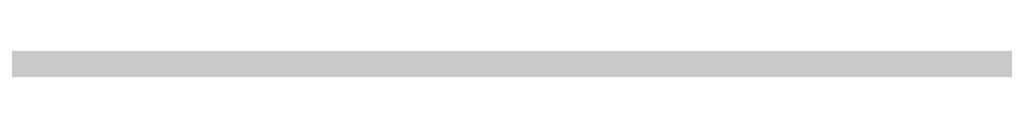
# Model space of a CAD drawing. Units: inches. Extents: x 2091 to 2899, y 967 to 2217.
# Tile 227 of 256: x 2203.4104 to 2203.7172, y 1152.2504 to 1152.2538. Entities that reach past the tile are written whole.
import ezdxf

# ---------------------------------------------------------------- set-up
doc = ezdxf.new("R2010")
doc.units = ezdxf.units.IN
doc.layers.add('A-WALL-PATT', color=141, linetype='Continuous', lineweight=13, true_color=0xadddf7)

msp = doc.modelspace()

# ---------------------------------------------------------------- hatches: boundary and pattern name
at = {"layer": 'A-WALL-PATT'}
h = msp.add_hatch(color=256, dxfattribs=at)
h.dxf.hatch_style = 1
h.paths.add_polyline_path([(2803.1436, 2050.91906), (2203.1436, 2050.91906), (2203.1436, 1090.91906), (2803.1436, 1090.91906)])
h.paths.add_polyline_path([(2635.79885, 1147.54046), (2674.52405, 1147.54046, 0.376086), (2678.52967, 1152.8802), (2678.52967, 1159.55647, 0.333335), (2674.52432, 1163.56185), (2674.52432, 1163.56185), (2674.52432, 1192.93439), (2635.80597, 1192.93439), (2597.08762, 1192.93439), (2597.08762, 1163.56185, 0.333335), (2593.08228, 1159.55647), (2593.08228, 1152.8802, 0.376086), (2597.08789, 1147.54046)], flags=0)
h.paths.add_polyline_path([(2436.01043, 1278.24078, 0.000483), (2435.95264, 1278.21503, -0.001328), (2435.93563, 1278.11169, -0.001711), (2436.11644, 1278.04076, 0.002185)], flags=0)
h.paths.add_polyline_path([(2794.1436, 1143.41906), (2794.1436, 1347.41906), (2543.37017, 1347.41906), (2543.37017, 1351.91906), (2794.1436, 1351.91906), (2794.1436, 1392.71355), (2793.9474, 1392.71355), (2793.9474, 1473.5369), (2794.1436, 1473.5369), (2794.1436, 1531.91906), (2650.1436, 1531.91906), (2650.1436, 1536.41906), (2794.1436, 1536.41906), (2794.1436, 1692.41906), (2609.37561, 1692.41906), (2609.37561, 1644.41906), (2604.87561, 1644.41906), (2604.87561, 1744.91906), (2609.37561, 1744.91906), (2609.37561, 1696.91906), (2794.1436, 1696.91906), (2794.1436, 1780.91906), (2609.6436, 1780.91906), (2493.87561, 1780.91906), (2493.87561, 1785.41906), (2609.6436, 1785.41906), (2794.1436, 1785.41906), (2794.1436, 1847.93882), (2793.95122, 1847.93882), (2793.95122, 1928.76217), (2794.1436, 1928.76217), (2794.1436, 1941.41906), (2614.1436, 1941.41906), (2614.1436, 1821.41906), (2609.6436, 1821.41906), (2609.6436, 1941.41906), (2392.1436, 1941.41906), (2392.1436, 1819.91906), (2387.6436, 1819.91906), (2387.6436, 1941.41906), (2212.1436, 1941.41906), (2212.1436, 1783.91906), (2392.1436, 1783.91906), (2392.1436, 1780.91906), (2212.1436, 1780.91906), (2212.1436, 1629.41906), (2387.6436, 1629.41906), (2387.6436, 1744.91906), (2392.1436, 1744.91906), (2392.1436, 1627.91906), (2317.1436, 1627.91906), (2317.1436, 1551.41906), (2317.1436, 1536.41906), (2459.38359, 1536.41906), (2459.38359, 1602.39648), (2463.88359, 1602.39648), (2463.88359, 1531.91906), (2456.6436, 1531.91906), (2456.6436, 1529.91906), (2452.1436, 1529.91906), (2452.1436, 1531.91906), (2312.6436, 1531.91906), (2312.6436, 1551.41906), (2306.1436, 1551.41906), (2306.1436, 1555.91906), (2308.1436, 1555.91906), (2308.1436, 1551.41906), (2312.6436, 1551.41906), (2312.6436, 1627.91906), (2212.1436, 1627.91906), (2212.1436, 1555.91906), (2270.1436, 1555.91906), (2270.1436, 1551.41906), (2212.1436, 1551.41906), (2212.1436, 1351.91906), (2272.1436, 1351.91906), (2272.1436, 1347.41906), (2212.1436, 1347.41906), (2212.1436, 1275.41906), (2308.1436, 1275.41906), (2308.1436, 1351.91906), (2452.1436, 1351.91906), (2452.1436, 1493.91906), (2456.6436, 1493.91906), (2456.6436, 1347.41906), (2312.6436, 1347.41906), (2312.6436, 1270.91906), (2212.1436, 1270.91906), (2212.1436, 1099.91906), (2281.23752, 1099.91906), (2282.87104, 1110.9138), (2282.00834, 1116.9966), (2278.55774, 1121.4204), (2268.20564, 1128.0562), (2272.08764, 1128.0562), (2273.81294, 1131.927), (2279.42034, 1134.6919), (2285.02784, 1135.2449), (2287.61584, 1137.4568), (2288.04714, 1138.0098), (2289.34114, 1140.7747), (2291.06654, 1139.6687), (2292.36054, 1135.2449), (2295.37984, 1136.9038), (2296.24254, 1135.7979), (2297.10524, 1133.033), (2300.12464, 1138.0098), (2303.14394, 1138.0098), (2304.43794, 1135.7979), (2303.14394, 1133.586), (2306.59464, 1134.6919), (2307.88874, 1133.033), (2310.90804, 1135.2449), (2313.92744, 1134.1389), (2315.62686, 1132.4271), (2308.32004, 1117.5496), (2290.20384, 1109.8079), (2288.90984, 1103.1721), (2289.27231, 1099.91906), (2434.91823, 1099.91906), (2431.59323, 1124.78806), (2429.93023, 1169.55306), (2430.92718, 1240.51969), (2435.65893, 1238.18613), (2437.13523, 1196.55406), (2438.79823, 1143.97306), (2442.67823, 1111.99806), (2446.55823, 1099.91906), (2794.1436, 1099.91906), (2794.1436, 1138.91906), (2548.03245, 1138.91906), (2548.03245, 1143.41906), (2548.03245, 1148.81906), (2546.66846, 1148.03156), (2528.68569, 1179.17862, 0.256256), (2512.03245, 1148.81906), (2512.03245, 1143.41906), (2512.03245, 1138.91906), (2507.53245, 1138.91906), (2507.53245, 1143.41906), (2507.53245, 1148.81906, 0.256256), (2490.8792, 1179.17862), (2472.89644, 1148.03156), (2471.53245, 1148.81906), (2471.53245, 1143.41906), (2467.03245, 1143.41906), (2467.03245, 1269.94579, 0.039061), (2460.90999, 1273.58006), (2467.03245, 1273.58006), (2467.03245, 1286.32536, 0.014511), (2465.21619, 1286.76191), (2467.03245, 1287.05258), (2467.03245, 1323.41906), (2471.53245, 1323.41906), (2471.53245, 1148.81906), (2489.53245, 1179.99597), (2490.89644, 1179.20847), (2490.8792, 1179.17862, -0.256256), (2507.53245, 1148.81906), (2507.53245, 1143.41906), (2512.03245, 1143.41906), (2512.03245, 1148.81906, -0.256256), (2528.68569, 1179.17862), (2528.66846, 1179.20847), (2530.03245, 1179.99597), (2548.03245, 1148.81906), (2548.03245, 1143.41906)], flags=16)
h.paths.add_polyline_path([(2607.76855, 1200.94508), (2607.76855, 1265.03063), (2597.08762, 1281.05201), (2619.78459, 1281.05201), (2627.79528, 1337.12686), (2635.79885, 1337.12686), (2643.81666, 1337.12686), (2651.82736, 1281.05201), (2674.52432, 1281.05201), (2663.8434, 1265.03063), (2663.8434, 1200.94508), (2635.80597, 1200.94508)], flags=0)
edge = h.paths.add_edge_path(flags=0)
edge.add_ellipse((13303.89622, 1272.99872), major_axis=(-10595.31304, 0), ratio=0.84230387009, start_angle=0.628237219, end_angle=0.6465541, ccw=False)
edge.add_ellipse((2711.70045, 1156.85268), major_axis=(2.21977, 0), ratio=0.8423039, start_angle=111.53524, end_angle=180.62824, ccw=False)
edge.add_ellipse((13303.15629, 1272.99872), major_axis=(-10593.02631, 0), ratio=0.84230386954, start_angle=0.528271472, end_angle=0.646554097, ccw=False)
edge.add_line((2710.7646, 1175.3333), (2710.12999, 1175.3333))
edge.add_ellipse((2710.12999, 1176.57978), major_axis=(1.47985, 0), ratio=0.8423039, start_angle=180, end_angle=270, ccw=False)
edge.add_line((2708.65014, 1176.57978), (2708.65014, 1200.78291))
edge.add_ellipse((2710.12999, 1200.78291), major_axis=(1.47985, 0), ratio=0.8423039, start_angle=90, end_angle=180, ccw=False)
edge.add_line((2710.12999, 1202.02939), (2710.46508, 1202.02939))
edge.add_ellipse((13303.15629, 1272.99872), major_axis=(-10593.02631, 0), ratio=0.84230386954, start_angle=-0.090229089, end_angle=0.383866779, ccw=False)
edge.add_ellipse((2710.12999, 1290.92703), major_axis=(-1.47985, 0), ratio=0.8423039, start_angle=0, end_angle=90, ccw=False)
edge.add_line((2708.65014, 1290.92703), (2708.65014, 1315.13017))
edge.add_ellipse((2710.12999, 1315.13017), major_axis=(-1.47985, 0), ratio=0.8423039, start_angle=-90, end_angle=0, ccw=False)
edge.add_line((2710.12999, 1316.37665), (2710.70631, 1316.37665))
edge.add_ellipse((3238.40172, 1296.28957), major_axis=(528.234, 0), ratio=0.84230387, start_angle=176.3495724, end_angle=177.8200497, ccw=False)
edge.add_ellipse((2775.06304, 1071.4507), major_axis=(313.30776, 0), ratio=0.84230387, start_angle=102.1259656, end_angle=103.780529, ccw=False)
edge.add_ellipse((2775.06304, 1078.3057), major_axis=(-305.30289, 0), ratio=0.84230387, start_angle=-79.790461, end_angle=-77.5553727, ccw=False)
edge.add_ellipse((2695.14177, 1541.97538), major_axis=(-250.96022, 0), ratio=0.84230387, start_angle=99.256566, end_angle=102.5549326)
edge.add_line((2741.41033, 1334.21426), (2747.13255, 1337.37848))
edge.add_ellipse((2747.53862, 1336.85748), major_axis=(-0.73992, 0), ratio=0.842304, start_angle=270, end_angle=307.93313, ccw=False)
edge.add_ellipse((2747.53862, 1336.85748), major_axis=(-0.73992, 0), ratio=0.842304, start_angle=232.06687, end_angle=270, ccw=False)
edge.add_line((2747.94469, 1337.37848), (2753.66691, 1334.21426))
edge.add_ellipse((2799.93547, 1541.97538), major_axis=(250.96022, 0), ratio=0.84230387, start_angle=257.4450674, end_angle=260.743434)
edge.add_ellipse((2720.01419, 1078.3057), major_axis=(305.30289, 0), ratio=0.84230387, start_angle=77.5553727, end_angle=79.790461, ccw=False)
edge.add_ellipse((2720.01419, 1071.4507), major_axis=(-313.30776, 0), ratio=0.84230387, start_angle=256.219471, end_angle=257.8740344, ccw=False)
edge.add_ellipse((2256.67551, 1296.28957), major_axis=(-528.234, 0), ratio=0.84230387, start_angle=182.1799503, end_angle=183.6504276, ccw=False)
edge.add_line((2784.37092, 1316.37665), (2784.94725, 1316.37665))
edge.add_ellipse((2784.94725, 1315.13017), major_axis=(1.47985, 0), ratio=0.8423039, start_angle=0, end_angle=90, ccw=False)
edge.add_line((2786.42709, 1315.13017), (2786.42709, 1290.92703))
edge.add_ellipse((2784.94725, 1290.92703), major_axis=(1.47985, 0), ratio=0.8423039, start_angle=270, end_angle=360, ccw=False)
edge.add_ellipse((-7808.07906, 1272.99872), major_axis=(10593.02631, 0), ratio=0.84230386954, start_angle=-0.383866779, end_angle=0.090229089, ccw=False)
edge.add_line((2784.61216, 1202.02939), (2784.94725, 1202.02939))
edge.add_ellipse((2784.94725, 1200.78291), major_axis=(1.47985, 0), ratio=0.8423039, start_angle=0, end_angle=90, ccw=False)
edge.add_line((2786.42709, 1200.78291), (2786.42709, 1176.57978))
edge.add_ellipse((2784.94725, 1176.57978), major_axis=(-1.47985, 0), ratio=0.8423039, start_angle=90, end_angle=180, ccw=False)
edge.add_line((2784.94725, 1175.3333), (2784.31264, 1175.3333))
edge.add_ellipse((-7808.07906, 1272.99872), major_axis=(10593.02631, 0), ratio=0.84230386954, start_angle=-0.618643196, end_angle=-0.528271472, ccw=False)
edge.add_ellipse((2783.37678, 1156.85268), major_axis=(-2.21977, 0), ratio=0.8423039, start_angle=179.37176, end_angle=248.46476, ccw=False)
edge.add_ellipse((-7808.81898, 1272.99872), major_axis=(-10595.31304, 0), ratio=0.84230386576, start_angle=179.353445923, end_angle=179.371762803, ccw=False)
edge.add_ellipse((2780.2973, 1153.50079), major_axis=(-5.24643, 0), ratio=0.8423039, start_angle=90, end_angle=179.35345, ccw=False)
edge.add_line((2780.2973, 1149.08171), (2714.77993, 1149.08171))
edge.add_ellipse((2714.77993, 1153.50079), major_axis=(5.24643, 0), ratio=0.8423039, start_angle=180.64655, end_angle=270, ccw=False)
edge = h.paths.add_edge_path(flags=0)
edge.add_line((2718.18737, 1151.00783), (2718.18737, 1170.47236))
edge.add_ellipse((2721.14706, 1170.47236), major_axis=(-2.95969, 0), ratio=0.8423039, start_angle=-90, end_angle=0, ccw=False)
edge.add_line((2721.14706, 1172.96532), (2773.93017, 1172.96532))
edge.add_ellipse((2773.93017, 1170.47236), major_axis=(-2.95969, 0), ratio=0.8423039, start_angle=180, end_angle=270, ccw=False)
edge.add_line((2776.88987, 1170.47236), (2776.88987, 1151.00783))
edge.add_line((2776.88987, 1151.00783), (2718.18737, 1151.00783))
edge = h.paths.add_edge_path(flags=0)
edge.add_line((2718.18737, 1180.23415), (2718.18737, 1199.05783))
edge.add_ellipse((2747.53862, 1320.39864), major_axis=(147.01792, 0), ratio=0.84230387, start_angle=256.4018653, end_angle=283.5981347)
edge.add_line((2776.88987, 1199.05783), (2776.88987, 1180.23415))
edge.add_ellipse((2747.53862, 1301.57496), major_axis=(147.01792, 0), ratio=0.84230387, start_angle=256.4018653, end_angle=283.5981347, ccw=False)
edge = h.paths.add_edge_path(flags=0)
edge.add_ellipse((13303.15629, 1272.99872), major_axis=(-10591.54646, 0), ratio=0.84230386955, start_angle=0.055594314, end_angle=0.377764194, ccw=False)
edge.add_line((2711.61686, 1262.72171), (2715.66741, 1249.4954))
edge.add_ellipse((6413.89196, 1241.69192), major_axis=(-3698.23616, 0), ratio=0.8423038695, start_angle=-0.12089737, end_angle=0.36407635)
edge.add_line((2715.76104, 1218.19245), (2711.93431, 1203.16736))
edge = h.paths.add_edge_path(flags=0)
edge.add_line((2718.18737, 1251.07457), (2716.00249, 1267.45044))
edge.add_ellipse((2742.15117, 1202.18954), major_axis=(81.77258, 0), ratio=0.84230387, start_angle=94.277421, end_angle=111.8349538, ccw=False)
edge.add_line((2737.00975, 1270.93063), (2758.06748, 1270.93063))
edge.add_ellipse((2752.92606, 1202.18954), major_axis=(81.77258, 0), ratio=0.84230387, start_angle=68.1650462, end_angle=85.722579, ccw=False)
edge.add_line((2779.07475, 1267.45044), (2776.88987, 1251.07457))
edge.add_ellipse((2750.33806, 1187.88536), major_axis=(79.57966, 0), ratio=0.84230387, start_angle=67.2080851, end_angle=85.1299304)
edge.add_line((2756.03466, 1254.74366), (2739.04258, 1254.74366))
edge.add_ellipse((2744.73917, 1187.88536), major_axis=(79.57966, 0), ratio=0.84230387, start_angle=94.8700696, end_angle=112.7919149)
edge = h.paths.add_edge_path(flags=0)
edge.add_line((2783.14293, 1203.16736), (2779.31619, 1218.19245))
edge.add_ellipse((-918.81473, 1241.69192), major_axis=(3698.23616, 0), ratio=0.8423038695, start_angle=-0.36407635, end_angle=0.12089737)
edge.add_line((2779.40983, 1249.4954), (2783.46037, 1262.72171))
edge.add_ellipse((-7808.07906, 1272.99872), major_axis=(-10591.54646, 0), ratio=0.84230386954, start_angle=179.622235806, end_angle=179.944405687, ccw=False)
edge = h.paths.add_edge_path(flags=0)
edge.add_ellipse((2734.20089, 1286.69044), major_axis=(-0.35661, 6.34008), ratio=0.6038336, start_angle=89.002014, end_angle=253.657408, ccw=False)
edge.add_line((2730.369, 1286.54181), (2730.369, 1301.35198))
edge.add_line((2730.369, 1301.35198), (2735.91331, 1305.2148))
edge.add_ellipse((2736.38492, 1304.73456), major_axis=(0.73992, 0), ratio=0.842304, start_angle=90, end_angle=134.48021, ccw=False)
edge.add_line((2736.38492, 1305.3578), (2738.03278, 1305.3578))
edge.add_line((2738.03278, 1305.3578), (2738.03278, 1307.70793))
edge.add_ellipse((2794.20164, 1307.70793), major_axis=(56.16886, 0), ratio=0.84230387, start_angle=150.56143, end_angle=180, ccw=False)
edge.add_ellipse((2700.87559, 1307.70793), major_axis=(-56.16886, 0), ratio=0.84230387, start_angle=180, end_angle=209.43857, ccw=False)
edge.add_line((2757.04445, 1307.70793), (2757.04445, 1305.3578))
edge.add_line((2757.04445, 1305.3578), (2758.69232, 1305.3578))
edge.add_ellipse((2758.69232, 1304.73456), major_axis=(-0.73992, 0), ratio=0.842304, start_angle=225.51979, end_angle=270, ccw=False)
edge.add_line((2759.16392, 1305.2148), (2764.70823, 1301.35198))
edge.add_line((2764.70823, 1301.35198), (2764.70823, 1286.54181))
edge.add_ellipse((2760.87634, 1286.69044), major_axis=(0.35661, 6.34008), ratio=0.6038336, start_angle=106.342592, end_angle=270.997986, ccw=False)
edge.add_line((2757.04445, 1285.79709), (2757.04445, 1307.70793))
edge.add_ellipse((2700.87559, 1307.70793), major_axis=(-56.16886, 0), ratio=0.84230387, start_angle=180, end_angle=209.43857)
edge.add_ellipse((2794.20164, 1307.70793), major_axis=(56.16886, 0), ratio=0.84230387, start_angle=150.56143, end_angle=180)
edge.add_line((2738.03278, 1307.70793), (2738.03278, 1285.79709))
h.paths.add_polyline_path([(2417.81227, 1104.4497), (2413.49227, 1102.5297), (2410.61227, 1103.9697), (2409.17227, 1106.3697), (2407.25227, 1107.3297), (2406.29227, 1109.7297), (2405.33227, 1114.0497), (2405.33227, 1117.8897), (2406.29227, 1120.1297), (2407.25227, 1119.8097), (2408.84832, 1118.32766), (2410.17395, 1119.42417), (2410.21127, 1120.4057), (2411.04073, 1121.41905), (2410.69927, 1119.8587), (2410.17395, 1119.42417), (2410.08845, 1117.17611), (2411.13284, 1116.20632), (2413.97227, 1119.3297), (2416.85227, 1120.7697), (2416.86972, 1120.79878), (2417.03507, 1119.40512), (2417.89621, 1118.14338), (2418.29227, 1118.3697), (2419.54445, 1120.03927), (2419.36092, 1118.38749), (2419.03211, 1119.35615), (2418.39894, 1118.51193), (2419.25227, 1114.5297), (2418.79409, 1107.19879)], flags=0)
h.paths.add_polyline_path([(2508.87017, 1347.41906), (2508.37017, 1347.41906), (2508.37017, 1351.91906), (2508.87017, 1351.91906)], flags=0)
h.paths.add_polyline_path([(2473.37017, 1347.41906), (2472.37017, 1347.41906), (2467.87017, 1347.41906), (2467.87017, 1455.41906), (2472.37017, 1455.41906), (2472.37017, 1352.41906), (2473.37017, 1352.41906)], flags=0)
h.paths.add_polyline_path([(2352.10624, 1217.4462), (2349.22624, 1218.8862), (2347.78624, 1221.2862), (2345.86624, 1222.2462), (2344.90624, 1224.6462), (2343.94624, 1228.9662), (2343.94624, 1232.8062), (2344.90624, 1235.0462), (2345.86624, 1234.7262), (2347.46229, 1233.24415), (2348.78792, 1234.34066), (2348.82524, 1235.3222), (2349.6547, 1236.33555), (2349.31324, 1234.7752), (2348.78792, 1234.34066), (2348.70242, 1232.0926), (2349.74681, 1231.12282), (2352.58624, 1234.2462), (2355.46624, 1235.6862), (2355.48369, 1235.71528), (2355.64904, 1234.32161), (2356.51018, 1233.05988), (2356.90624, 1233.2862), (2358.15842, 1234.95576), (2357.97489, 1233.30398), (2357.64608, 1234.27264), (2357.01291, 1233.42842), (2357.86624, 1229.4462), (2357.40806, 1222.11529), (2356.42624, 1219.3662)], flags=0)
h.paths.add_polyline_path([(2348.2968, 1112.22442), (2347.0138, 1112.31042), (2345.5298, 1114.12742), (2345.7318, 1115.85842), (2346.8118, 1116.98242), (2346.8118, 1114.64642), (2345.8668, 1114.21442), (2346.8798, 1114.30042)], flags=0)
h.paths.add_polyline_path([(2347.0138, 1110.92642), (2346.2718, 1110.49342), (2346.6098, 1111.18642)], flags=0)
h.paths.add_polyline_path([(2345.8668, 1118.19442), (2345.5298, 1117.32942), (2343.7078, 1118.02142), (2344.3828, 1118.62642)], flags=0)
h.paths.add_polyline_path([(2346.6768, 1109.28242), (2346.0698, 1108.07142), (2345.8668, 1110.06142)], flags=0)
h.paths.add_polyline_path([(2345.0568, 1119.75142), (2343.6398, 1119.75142), (2343.9778, 1121.13542)], flags=0)
h.paths.add_polyline_path([(2345.2598, 1116.55042), (2345.1248, 1115.85842), (2344.9218, 1115.68542), (2344.7198, 1116.37742)], flags=0)
h.paths.add_polyline_path([(2345.6648, 1112.31042), (2345.4618, 1111.53242), (2344.0448, 1111.96442), (2344.6518, 1112.57042)], flags=0)
h.paths.add_polyline_path([(2345.1918, 1113.34942), (2344.4498, 1113.86842), (2344.7198, 1114.38742)], flags=0)
h.paths.add_polyline_path([(2344.6518, 1116.80942), (2344.1798, 1115.68542), (2344.6518, 1115.33942), (2343.9098, 1114.90642), (2343.0328, 1115.94442), (2343.6398, 1116.46342)], flags=0)
h.paths.add_polyline_path([(2345.8668, 1106.68642), (2344.9898, 1105.56242), (2344.5168, 1106.60042)], flags=0)
h.paths.add_polyline_path([(2344.8548, 1110.06142), (2344.5168, 1109.28242), (2344.1128, 1109.71542)], flags=0)
h.paths.add_polyline_path([(2344.0448, 1113.52242), (2343.4378, 1113.08942), (2342.7628, 1113.95442)], flags=0)
h.paths.add_polyline_path([(2344.3148, 1111.01242), (2342.9648, 1110.32042), (2342.9648, 1111.09942)], flags=0)
h.paths.add_polyline_path([(2345.1248, 1104.69742), (2344.5848, 1103.74542), (2344.4498, 1104.26442)], flags=0)
h.paths.add_polyline_path([(2342.8298, 1121.22242), (2341.7498, 1120.53042), (2340.5358, 1121.04942), (2340.1308, 1121.82842), (2340.6708, 1122.95242), (2341.1428, 1121.82842), (2341.6148, 1122.00142)], flags=0)
h.paths.add_polyline_path([(2342.9648, 1119.75142), (2343.0328, 1118.45342), (2342.0878, 1118.02142), (2342.0198, 1119.49142)], flags=0)
h.paths.add_polyline_path([(2342.6948, 1116.89642), (2341.9528, 1116.63642), (2342.0198, 1117.32942)], flags=0)
h.paths.add_polyline_path([(2343.0328, 1112.22442), (2342.0198, 1111.79142), (2341.5478, 1112.22442), (2342.3578, 1113.34942)], flags=0)
h.paths.add_polyline_path([(2343.7748, 1104.43742), (2342.6278, 1102.88042), (2342.6948, 1104.61042), (2343.4378, 1105.12942)], flags=0)
h.paths.add_polyline_path([(2342.0198, 1115.07942), (2340.8058, 1115.51242), (2340.9408, 1116.37742)], flags=0)
h.paths.add_polyline_path([(2341.4808, 1120.09742), (2341.4808, 1119.40542), (2341.0758, 1119.57842), (2341.1428, 1120.09742)], flags=0)
h.paths.add_polyline_path([(2341.8178, 1114.47342), (2340.9408, 1113.08942), (2340.8058, 1114.56042)], flags=0)
h.paths.add_polyline_path([(2341.1428, 1118.54042), (2340.9408, 1116.98242), (2339.0508, 1117.67542), (2339.0508, 1118.62642)], flags=0)
h.paths.add_polyline_path([(2342.6948, 1101.66842), (2341.9528, 1101.84142), (2342.5598, 1102.36142)], flags=0)
h.paths.add_polyline_path([(2340.3328, 1119.66542), (2338.4438, 1119.57842), (2337.9038, 1120.35742), (2339.6578, 1120.61642)], flags=0)
h.paths.add_polyline_path([(2340.3328, 1115.33942), (2340.0628, 1113.69542), (2339.3878, 1115.33942)], flags=0)
h.paths.add_polyline_path([(2341.8178, 1103.83142), (2341.5478, 1102.88042), (2341.1428, 1103.65842)], flags=0)
h.paths.add_polyline_path([(2339.0508, 1122.86642), (2337.2958, 1121.82842), (2337.0938, 1123.12542), (2337.7688, 1123.81842)], flags=0)
h.paths.add_polyline_path([(2339.1178, 1121.74142), (2338.8478, 1121.22242), (2338.1738, 1121.04942), (2338.3758, 1121.56842)], flags=0)
h.paths.add_polyline_path([(2339.1858, 1119.31942), (2338.6458, 1118.71342), (2338.2408, 1118.10742), (2338.2408, 1118.88642)], flags=0)
h.paths.add_polyline_path([(2341.1428, 1101.92842), (2340.6028, 1101.23642), (2340.0628, 1101.84142), (2340.6028, 1102.36142)], flags=0)
h.paths.add_polyline_path([(2337.6338, 1117.76142), (2336.6208, 1118.28042), (2337.2958, 1118.97242)], flags=0)
h.paths.add_polyline_path([(2336.8238, 1119.57842), (2334.7988, 1118.97242), (2335.2038, 1120.35742), (2336.5538, 1120.87642)], flags=0)
h.paths.add_polyline_path([(2339.1178, 1100.45742), (2337.3638, 1100.54342), (2336.7558, 1101.23642)], flags=0)
h.paths.add_polyline_path([(2336.3508, 1122.43342), (2336.0138, 1121.91442), (2334.9338, 1122.43342), (2334.5288, 1123.47142), (2335.7438, 1122.77942)], flags=0)
h.paths.add_polyline_path([(2334.7318, 1120.87642), (2334.2588, 1120.35742), (2334.0568, 1120.78942), (2334.5968, 1121.30842)], flags=0)
h.paths.add_polyline_path([(2334.4618, 1122.17442), (2332.5718, 1121.30842), (2331.3568, 1122.17442), (2332.0998, 1122.86642)], flags=0)
h.paths.add_polyline_path([(2334.2588, 1118.54042), (2333.3818, 1118.45342), (2333.6518, 1119.31942)], flags=0)
h.paths.add_polyline_path([(2335.5418, 1102.27442), (2334.1918, 1102.62042), (2335.2718, 1103.31242)], flags=0)
h.paths.add_polyline_path([(2332.7068, 1119.66542), (2331.6948, 1120.44342), (2332.5048, 1120.78942)], flags=0)
h.paths.add_polyline_path([(2334.7318, 1101.14942), (2333.5168, 1101.58242), (2333.9888, 1101.75542)], flags=0)
h.paths.add_polyline_path([(2332.6398, 1116.63642), (2331.0868, 1116.29042), (2331.9648, 1118.19442)], flags=0)
h.paths.add_polyline_path([(2330.7498, 1121.56842), (2330.2768, 1120.27042), (2328.5228, 1119.31942), (2328.9948, 1121.04942)], flags=0)
h.paths.add_polyline_path([(2330.7498, 1118.62642), (2330.0078, 1117.50242), (2329.8728, 1118.02142)], flags=0)
h.paths.add_polyline_path([(2332.0998, 1102.36142), (2330.5468, 1102.01442), (2331.6948, 1102.96642)], flags=0)
h.paths.add_polyline_path([(2329.5348, 1113.60842), (2329.0628, 1112.31042), (2328.5898, 1113.34942)], flags=0)
h.paths.add_polyline_path([(2328.3878, 1117.84842), (2327.5098, 1116.55042), (2327.1728, 1117.76142)], flags=0)
h.paths.add_polyline_path([(2329.7378, 1106.51342), (2329.5348, 1105.30242), (2328.2528, 1106.08142)], flags=0)
h.paths.add_polyline_path([(2328.6578, 1114.38742), (2328.0498, 1114.12742), (2328.3198, 1114.90642)], flags=0)
h.paths.add_polyline_path([(2328.3198, 1112.22442), (2327.1058, 1112.13742), (2326.7008, 1112.65642)], flags=0)
h.paths.add_polyline_path([(2326.9028, 1115.25242), (2326.7008, 1114.12742), (2325.2158, 1113.60842), (2326.0928, 1115.33942)], flags=0)
h.paths.add_polyline_path([(2326.6328, 1108.33042), (2326.0928, 1107.37942), (2325.8908, 1108.50342), (2326.4978, 1109.10942)], flags=0)
h.paths.add_polyline_path([(2615.1436, 1531.91906), (2609.6436, 1531.91906), (2609.6436, 1620.41906), (2614.1436, 1620.41906), (2614.1436, 1536.41906), (2615.1436, 1536.41906)], flags=0)
h.paths.add_polyline_path([(2545.1436, 1563.41906), (2464.1436, 1563.41906), (2464.1436, 1632.41906), (2509.1436, 1632.41906), (2509.1436, 1627.91906), (2509.1436, 1603.91906), (2468.6436, 1603.91906), (2468.6436, 1567.91906), (2540.6436, 1567.91906), (2540.6436, 1591.91906), (2545.1436, 1591.91906)], flags=0)
h.paths.add_polyline_path([(2388.96905, 1549.98573), (2357.43418, 1549.98573), (2357.43418, 1623.36078), (2399.36278, 1623.36078), (2435.68947, 1623.36078), (2435.59255, 1602.55927), (2435.59255, 1602.39648), (2388.96905, 1602.39648)], flags=0)
h.paths.add_polyline_path([(2388.88063, 1555.80915), (2374.90443, 1555.80915), (2374.90443, 1600.57156), (2374.90443, 1615.45765), (2406.35088, 1615.45765), (2406.35088, 1618.93943), (2412.17429, 1615.45765), (2406.35088, 1611.97586), (2406.35088, 1615.45765), (2388.88063, 1615.45765)], flags=0)
h.paths.add_polyline_path([(2568.87561, 1644.41906), (2453.37561, 1644.41906), (2453.37561, 1785.41906), (2457.87561, 1785.41906), (2457.87561, 1648.91906), (2568.87561, 1648.91906)], flags=0)
h.paths.add_polyline_path([(2212.1436, 1945.91906), (2212.1436, 2041.91906), (2794.1436, 2041.91906), (2794.1436, 1945.91906)], flags=16)
h.paths.add_polyline_path([(2271.08273, 1964.31724), (2776.85297, 1964.31724), (2776.85297, 2037.16962), (2271.08273, 2037.16962)], flags=8)
h.paths.add_polyline_path([(2380.64929, 1536.82414), (2461.04081, 1536.82414), (2461.04081, 1554.65259), (2380.64929, 1554.65259)], flags=8)
h.paths.add_polyline_path([(2240.75571, 1609.72545), (2309.18583, 1609.72545), (2309.18583, 1617.6982), (2240.75571, 1617.6982)], flags=8)
h.paths.add_polyline_path([(2212.67726, 1313.5041), (2282.59152, 1313.5041), (2282.59152, 1322.74524), (2212.67726, 1322.74524)], flags=8)
h.paths.add_polyline_path([(2457.11198, 1114.77857), (2558.48158, 1114.77857), (2558.48158, 1142.21968), (2457.11198, 1142.21968)], flags=8)
h.paths.add_polyline_path([(2473.44234, 1273.01007), (2604.64123, 1273.01007), (2604.64123, 1318.34693), (2473.44234, 1318.34693)], flags=8)
h.paths.add_polyline_path([(2638.8763, 1626.97743), (2684.25037, 1627.97674), (2684.03848, 1637.59749), (2638.66442, 1636.59819)], flags=8)
h.paths.add_polyline_path([(2537.59055, 1453.79345), (2628.38955, 1453.79345), (2628.38955, 1475.34481), (2537.59055, 1475.34481)], flags=8)
h.paths.add_polyline_path([(2504.13764, 1714.6324), (2554.64719, 1714.6324), (2554.64719, 1730.23771), (2504.13764, 1730.23771)], flags=8)
h.paths.add_polyline_path([(2487.50118, 1575.65187), (2535.09712, 1575.65187), (2535.09712, 1598.37765), (2487.50118, 1598.37765)], flags=8)
h.paths.add_polyline_path([(2709.0994, 1735.71028), (2740.0166, 1735.71028), (2740.0166, 1749.93764), (2709.0994, 1749.93764)], flags=8)
h.paths.add_polyline_path([(2442.43842, 1792.17166), (2564.72884, 1792.17166), (2564.72884, 1842.00016), (2442.43842, 1842.00016)], flags=8)
h.paths.add_polyline_path([(2655.8158, 1809.64408), (2789.52014, 1806.6938), (2790.08498, 1832.29164), (2656.38064, 1835.24192)], flags=8)
h.paths.add_polyline_path([(2234.8427, 1797.72014), (2368.59285, 1794.76885), (2369.16072, 1820.50413), (2235.41056, 1823.45542)], flags=8)
h.paths.add_polyline_path([(2245.13847, 1644.00633), (2398.42773, 1640.6239), (2398.99484, 1666.32482), (2245.70557, 1669.70725)], flags=8)
h.paths.add_polyline_path([(2306.14285, 1431.16852), (2413.76831, 1428.79369), (2414.33315, 1454.39153), (2306.70768, 1456.76636)], flags=8)
h.paths.add_polyline_path([(2306.83458, 1458.23314), (2393.38048, 1456.32345), (2393.93281, 1481.35436), (2307.38691, 1483.26405)], flags=8)

doc.saveas('drawing.dxf')
